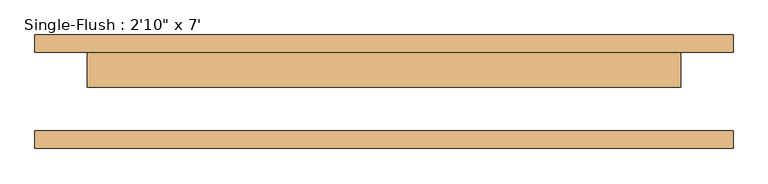
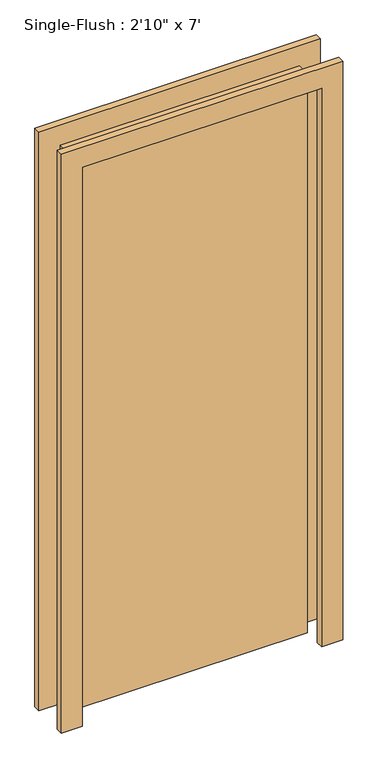
"""IFC4 building model written with IfcOpenShell, lengths in millimetres: door geometry."""

from ifc_helpers import new_model, si_unit, frame, origin, origin_with_axes, place, context, project, spatial, polyline, outline, extrude, source, transform, mapped, element, save


def door_70e57c00(model_context):
    return source(origin(), model_context, "Body", "SweptSolid", [
        extrude(outline(polyline([(2209.8, -508.0), (0.0, -508.0), (0.0, -431.8), (2133.6, -431.8), (2133.6, 431.8), (0.0, 431.8), (0.0, 508.0), (2209.8, 508.0), (2209.8, -508.0)])), frame((0.0, 57.15, 0.0), z_axis=(0.0, 1.0, 0.0), x_axis=(0.0, 0.0, 1.0)), (0.0, 0.0, 1.0), 25.4),
        extrude(outline(polyline([(2209.8, 508.0), (2209.8, -508.0), (0.0, -508.0), (0.0, -431.8), (2133.6, -431.8), (2133.6, 431.8), (0.0, 431.8), (0.0, 508.0), (2209.8, 508.0)])), frame((0.0, -82.55, 0.0), z_axis=(0.0, 1.0, 0.0), x_axis=(0.0, 0.0, 1.0)), (0.0, 0.0, 1.0), 25.4),
        extrude(outline(polyline([(431.8, 6.35), (-431.8, 6.35), (-431.8, 57.15), (431.8, 57.15), (431.8, 6.35)])), origin_with_axes(), (0.0, 0.0, 1.0), 2133.6),
    ])


if __name__ == "__main__":
    model = new_model("IFC4")
    model_context = context("Model", 3, world=origin())
    ifc_project = project(units=[si_unit("LENGTHUNIT", "METRE", prefix="MILLI")], contexts=[model_context])
    site = spatial("IfcSite", under=ifc_project)
    building = spatial("IfcBuilding", under=site)
    placement = place(None, origin())
    door_shape = door_70e57c00(model_context)
    element("IfcDoor", 1, ObjectType="Single-Flush : 2'10\" x 7'", at=placement, inside=building, context=model_context, shape_type="MappedRepresentation", body=[
        mapped(door_shape, transform((0.0, 0.0, 0.0), x_axis=(1.0, 0.0, 0.0), y_axis=(0.0, 1.0, 0.0), z_axis=(0.0, 0.0, 1.0))),
    ])
    save(model, "model.ifc")

# Revit data of these elements
# Type "Single-Flush : 2'10\" x 7'"
#   Type Mark = "13"
#   Construction Type Id = "MDOOR"
#   Assembly Code = "C1020"
#   Analytic Construction = "Metal"
#   Thickness = 0' - 2"
#   Heat Transfer Coefficient (U) = 0.651978 BTU/(h·ft²·°F)
#   Height = 7' - 0"
#   Trim Projection Ext = 0' - 1"
#   Trim Projection Int = 0' - 1"
#   Trim Width = 0' - 3"
#   Width = 2' - 10"
#   Define Thermal Properties by = 1
#   Door Material = Door - Panel
#   Frame Material = Door - Frame
#   Visual Light Transmittance = 0
#   Solar Heat Gain Coefficient = 0
#   Function = (empty or 0)
#   Wall Closure = (empty or 0)
# Element 1 (IfcDoor, "Single-Flush : 2'10\" x 7'")
#   Materials on its faces: "Door - Frame", "Door - Panel"
# Materials
#   "Door - Panel": class "Wood", colour RGB 210 159 95, transparency 0, Cost = 0
#   "Door - Frame": colour RGB 118 70 51, transparency 0, Cost = 0
